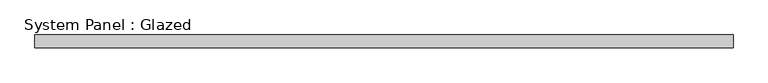
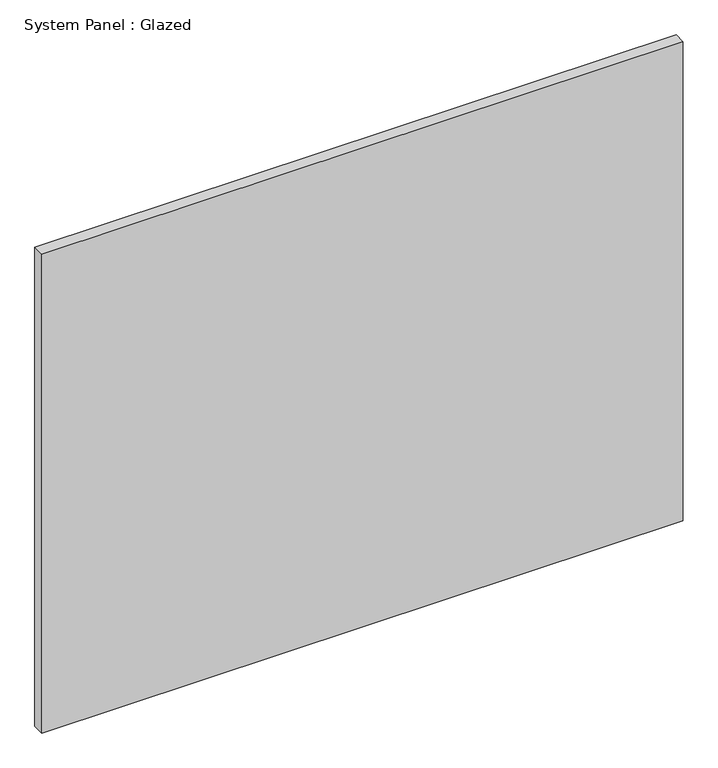
"""IFC4 building model written with IfcOpenShell, lengths in millimetres: plate geometry, System Panel : Glazed."""

from ifc_helpers import new_model, si_unit, origin, origin_with_axes, place, context, project, spatial, polyline, outline, extrude, source, transform, mapped, element, save


def system_panel_glazed_e0df8542(model_context):
    return source(origin(), model_context, "Body", "SweptSolid", [
        extrude(outline(polyline([(692.15, 19.05), (-692.15, 19.05), (-692.15, 44.45), (692.15, 44.45), (692.15, 19.05)])), origin_with_axes(), (0.0, 0.0, 1.0), 1092.2),
    ])


if __name__ == "__main__":
    model = new_model("IFC4")
    model_context = context("Model", 3, world=origin())
    ifc_project = project(units=[si_unit("LENGTHUNIT", "METRE", prefix="MILLI")], contexts=[model_context])
    site = spatial("IfcSite", under=ifc_project)
    building = spatial("IfcBuilding", under=site)
    placement = place(None, origin())
    system_panel_glazed_shape = system_panel_glazed_e0df8542(model_context)
    element("IfcPlate", 1, ObjectType="System Panel : Glazed", at=placement, inside=building, context=model_context, shape_type="MappedRepresentation", body=[
        mapped(system_panel_glazed_shape, transform((0.0, 0.0, 0.0), x_axis=(1.0, 0.0, 0.0), y_axis=(0.0, 1.0, 0.0), z_axis=(0.0, 0.0, 1.0))),
    ])
    save(model, "model.ifc")

# Revit data of these elements
# Type "System Panel : Glazed"
#   Construction Type Id = "GSP4R"
#   Analytic Construction = "1/8 in Pilkington single glazing"
#   Visual Light Transmittance = 0.9
#   Solar Heat Gain Coefficient = 0.86
#   Heat Transfer Coefficient (U) = 1.18115 BTU/(h·ft²·°F)
#   Define Thermal Properties by = 1
# Element 1 (IfcPlate, "System Panel : Glazed")
#   Materials on its faces: "Glass"
# Materials
#   "Glass": class "Glass", colour RGB 0 128 192, transparency 0.75, Description = "Soda Lime Glass", Cost = 0
